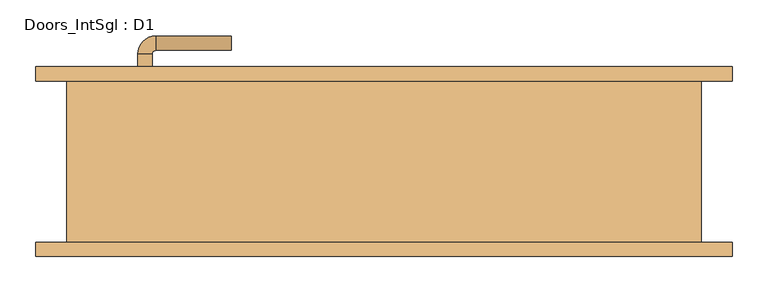
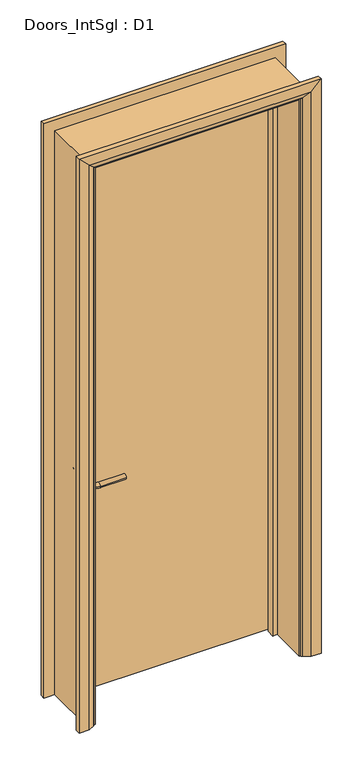
"""IFC4 building model written with IfcOpenShell, lengths in millimetres: door geometry, Doors_IntSgl : D1."""

from ifc_helpers import new_model, si_unit, point, frame, frame_2d, origin, place, context, project, spatial, polyline, circle_curve, ellipse_curve, trimmed, segment, composite_curve, outline, extrude, faceted_brep, source, transform, mapped, element, save
from ifc_brep_helpers import plane_surface, cylinder_surface, revolved_surface, advanced_brep


def doors_intsgl_d1_267d61ee(model_context):
    return source(origin(), model_context, "Body", "SolidModel", [
        advanced_brep(
        [(-343.0, 66.5, 900.0), (-323.0, 66.5, 900.0), (-323.0, 36.5, 900.0), (-343.0, 36.5, 900.0), (-318.0, 31.5, 900.0), (-318.0, 11.5, 900.0), (-213.0, 11.5, 900.0), (-213.0, 31.5, 900.0)],
        [
            (0, 1, circle_curve(frame((-333.0, 66.5, 900.0), z_axis=(0.0, 1.0, 0.0), x_axis=(1.0, 0.0, 0.0)), 10.0)),
            (1, 0, circle_curve(frame((-333.0, 66.5, 900.0), z_axis=(0.0, 1.0, 0.0), x_axis=(1.0, 0.0, 0.0)), 10.0)),
            (1, 2),
            (2, 3, circle_curve(frame((-333.0, 36.5, 900.0), z_axis=(0.0, 1.0, 0.0), x_axis=(1.0, 0.0, 0.0)), 10.0)),
            (3, 0),
            (3, 2, circle_curve(frame((-333.0, 36.5, 900.0), z_axis=(0.0, 1.0, 0.0), x_axis=(1.0, 0.0, 0.0)), 10.0)),
            (4, 5, circle_curve(frame((-318.0, 21.5, 900.0), z_axis=(-1.0, 0.0, 0.0), x_axis=(0.0, 1.0, 0.0)), 10.0)),
            (5, 3, circle_curve(frame((-318.0, 36.5, 900.0), z_axis=(0.0, 0.0, -1.0), x_axis=(-1.0, 0.0, 0.0)), 25.0)),
            (2, 4, circle_curve(frame((-318.0, 36.5, 900.0), z_axis=(0.0, 0.0, 1.0), x_axis=(-1.0, 0.0, 0.0)), 5.0)),
            (5, 4, circle_curve(frame((-318.0, 21.5, 900.0), z_axis=(-1.0, 0.0, 0.0), x_axis=(0.0, 1.0, 0.0)), 10.0)),
            (6, 7, circle_curve(frame((-213.0, 21.5, 900.0), z_axis=(1.0, 0.0, 0.0), x_axis=(0.0, 1.0, 0.0)), 10.0)),
            (7, 6, circle_curve(frame((-213.0, 21.5, 900.0), z_axis=(1.0, 0.0, 0.0), x_axis=(0.0, 1.0, 0.0)), 10.0)),
            (4, 7),
            (6, 5),
        ],
        [
            plane_surface(frame((-333.0, 66.5, 900.0), z_axis=(0.0, 1.0, 0.0), x_axis=(0.0, 0.0, 1.0))),
            cylinder_surface(frame((-333.0, 66.5, 900.0), z_axis=(0.0, 1.0, 0.0), x_axis=(1.0, 0.0, 0.0)), 10.0),
            revolved_surface(trimmed(ellipse_curve(frame((-333.0, 36.5, 900.0), z_axis=(0.0, -1.0, 0.0), x_axis=(1.0, 0.0, 0.0)), 10.0, 10.0), [point((-343.0, 36.5, 900.0))], [point((-323.0, 36.5, 900.0))], True, "CARTESIAN"), (-318.0, 36.5, 900.0), (0.0, 0.0, -1.0)),
            revolved_surface(trimmed(ellipse_curve(frame((-333.0, 36.5, 900.0), z_axis=(0.0, -1.0, 0.0), x_axis=(1.0, 0.0, 0.0)), 10.0, 10.0), [point((-323.0, 36.5, 900.0))], [point((-343.0, 36.5, 900.0))], True, "CARTESIAN"), (-318.0, 36.5, 900.0), (0.0, 0.0, -1.0)),
            plane_surface(frame((-213.0, 21.5, 900.0), z_axis=(1.0, 0.0, 0.0), x_axis=(0.0, 0.0, 1.0))),
            cylinder_surface(frame((-318.0, 21.5, 900.0), z_axis=(-1.0, 0.0, 0.0), x_axis=(0.0, 1.0, 0.0)), 10.0),
        ],
        [
            (0, [[1, 2]]),
            (1, [[3, 4, 5, -2]]),
            (1, [[-5, 6, -3, -1]]),
            (2, [[7, 8, -4, 9]]),
            (3, [[10, -9, -6, -8]]),
            (4, [[11, 12]]),
            (5, [[13, -11, 14, -7]]),
            (5, [[-14, -12, -13, -10]]),
        ],
    ),
        extrude(outline(composite_curve([segment(trimmed(circle_curve(frame_2d((900.0, -335.5)), 30.0), [point((900.0, -365.5))], [point((900.0, -305.5))], False, "CARTESIAN"), True, "CONTINUOUS"), segment(trimmed(circle_curve(frame_2d((900.0, -335.5)), 30.0), [point((900.0, -305.5))], [point((900.0, -365.5))], False, "CARTESIAN"), True, "CONTINUOUS")], self_intersect=False)), frame((0.0, 66.5, 0.0), z_axis=(0.0, 1.0, 0.0), x_axis=(0.0, 0.0, 1.0)), (0.0, 0.0, 1.0), 8.0),
        advanced_brep(
        [(-343.0, 120.5, 900.0), (-323.0, 120.5, 900.0), (-343.0, 150.5, 900.0), (-323.0, 150.5, 900.0), (-318.0, 155.5, 900.0), (-318.0, 175.5, 900.0), (-213.0, 175.5, 900.0), (-213.0, 155.5, 900.0)],
        [
            (0, 1, circle_curve(frame((-333.0, 120.5, 900.0), z_axis=(0.0, -1.0, 0.0), x_axis=(1.0, 0.0, 0.0)), 10.0)),
            (1, 0, circle_curve(frame((-333.0, 120.5, 900.0), z_axis=(0.0, -1.0, 0.0), x_axis=(1.0, 0.0, 0.0)), 10.0)),
            (0, 2),
            (2, 3, circle_curve(frame((-333.0, 150.5, 900.0), z_axis=(0.0, -1.0, 0.0), x_axis=(1.0, 0.0, 0.0)), 10.0)),
            (3, 1),
            (3, 2, circle_curve(frame((-333.0, 150.5, 900.0), z_axis=(0.0, -1.0, 0.0), x_axis=(1.0, 0.0, 0.0)), 10.0)),
            (4, 3, circle_curve(frame((-318.0, 150.5, 900.0), z_axis=(0.0, 0.0, 1.0), x_axis=(-1.0, 0.0, 0.0)), 5.0)),
            (2, 5, circle_curve(frame((-318.0, 150.5, 900.0), z_axis=(0.0, 0.0, -1.0), x_axis=(-1.0, 0.0, 0.0)), 25.0)),
            (5, 4, circle_curve(frame((-318.0, 165.5, 900.0), z_axis=(-1.0, 0.0, 0.0), x_axis=(0.0, -1.0, 0.0)), 10.0)),
            (4, 5, circle_curve(frame((-318.0, 165.5, 900.0), z_axis=(-1.0, 0.0, 0.0), x_axis=(0.0, -1.0, 0.0)), 10.0)),
            (6, 7, circle_curve(frame((-213.0, 165.5, 900.0), z_axis=(1.0, 0.0, 0.0), x_axis=(0.0, -1.0, 0.0)), 10.0)),
            (7, 6, circle_curve(frame((-213.0, 165.5, 900.0), z_axis=(1.0, 0.0, 0.0), x_axis=(0.0, -1.0, 0.0)), 10.0)),
            (5, 6),
            (7, 4),
        ],
        [
            plane_surface(frame((-333.0, 120.5, 900.0), z_axis=(0.0, -1.0, 0.0), x_axis=(0.0, 0.0, 1.0))),
            cylinder_surface(frame((-333.0, 120.5, 900.0), z_axis=(0.0, -1.0, 0.0), x_axis=(1.0, 0.0, 0.0)), 10.0),
            revolved_surface(trimmed(ellipse_curve(frame((-333.0, 150.5, 900.0), z_axis=(0.0, -1.0, 0.0), x_axis=(1.0, 0.0, 0.0)), 10.0, 10.0), [point((-343.0, 150.5, 900.0))], [point((-323.0, 150.5, 900.0))], True, "CARTESIAN"), (-318.0, 150.5, 900.0), (0.0, 0.0, -1.0)),
            revolved_surface(trimmed(ellipse_curve(frame((-333.0, 150.5, 900.0), z_axis=(0.0, -1.0, 0.0), x_axis=(1.0, 0.0, 0.0)), 10.0, 10.0), [point((-323.0, 150.5, 900.0))], [point((-343.0, 150.5, 900.0))], True, "CARTESIAN"), (-318.0, 150.5, 900.0), (0.0, 0.0, -1.0)),
            plane_surface(frame((-213.0, 165.5, 900.0), z_axis=(1.0, 0.0, 0.0), x_axis=(0.0, 0.0, 1.0))),
            cylinder_surface(frame((-318.0, 165.5, 900.0), z_axis=(-1.0, 0.0, 0.0), x_axis=(0.0, -1.0, 0.0)), 10.0),
        ],
        [
            (0, [[1, 2]]),
            (1, [[-1, 3, 4, 5]]),
            (1, [[-2, -5, 6, -3]]),
            (2, [[7, -4, 8, 9]]),
            (3, [[-8, -6, -7, 10]]),
            (4, [[11, 12]]),
            (5, [[-9, 13, -12, 14]]),
            (5, [[-10, -14, -11, -13]]),
        ],
    ),
        extrude(outline(composite_curve([segment(trimmed(circle_curve(frame_2d((900.0, -335.5)), 30.0), [point((900.0, -365.5))], [point((900.0, -305.5))], False, "CARTESIAN"), True, "CONTINUOUS"), segment(trimmed(circle_curve(frame_2d((900.0, -335.5)), 30.0), [point((900.0, -305.5))], [point((900.0, -365.5))], False, "CARTESIAN"), True, "CONTINUOUS")], self_intersect=False)), frame((0.0, 112.5, 0.0), z_axis=(0.0, 1.0, 0.0), x_axis=(0.0, 0.0, 1.0)), (0.0, 0.0, 1.0), 8.0),
        extrude(outline(polyline([(408.0, 74.5), (-408.0, 74.5), (-408.0, 112.5), (408.0, 112.5), (408.0, 74.5)])), frame((0.0, 0.0, 8.0), z_axis=(0.0, 0.0, 1.0), x_axis=(1.0, 0.0, 0.0)), (0.0, 0.0, 1.0), 2350.0),
        faceted_brep([(-410.0, 112.5, 0.0), (-410.0, -112.5, 0.0), (-442.0, -112.5, 0.0), (-442.0, 112.5, 0.0), (-410.0, 112.5, 2360.0), (-410.0, -112.5, 2360.0), (-442.0, -112.5, 2392.0), (-442.0, 112.5, 2392.0), (410.0, 112.5, 0.0), (442.0, 112.5, 0.0), (442.0, -112.5, 0.0), (410.0, -112.5, 0.0), (410.0, 112.5, 2360.0), (442.0, 112.5, 2392.0), (442.0, -112.5, 2392.0), (410.0, -112.5, 2360.0)], [[[0, 1, 2, 3]], [[1, 0, 4, 5]], [[2, 1, 5, 6]], [[3, 2, 6, 7]], [[0, 3, 7, 4]], [[8, 9, 10, 11]], [[12, 13, 9, 8]], [[13, 14, 10, 9]], [[14, 15, 11, 10]], [[15, 12, 8, 11]], [[5, 4, 12, 15]], [[6, 5, 15, 14]], [[7, 6, 14, 13]], [[4, 7, 13, 12]]]),
        advanced_brep(
        [(-485.0, -132.5, 0.0), (-485.0, -112.5, 0.0), (-415.0, -112.5, 0.0), (-419.0, -118.5, 0.0), (-445.0, -132.5, 0.0), (-485.0, -132.5, 2435.0), (-485.0, -112.5, 2435.0), (-415.0, -112.5, 2365.0), (-419.0, -118.5, 2369.0), (-445.0, -132.5, 2395.0), (485.0, -132.5, 0.0), (445.0, -132.5, 0.0), (419.0, -118.5, 0.0), (415.0, -112.5, 0.0), (485.0, -112.5, 0.0), (485.0, -132.5, 2435.0), (445.0, -132.5, 2395.0), (419.0, -118.5, 2369.0), (415.0, -112.5, 2365.0), (485.0, -112.5, 2435.0)],
        [
            (0, 1),
            (1, 2),
            (2, 3, circle_curve(frame((-423.0, -111.5, 0.0), z_axis=(0.0, 0.0, -1.0), x_axis=(-1.0, 0.0, 0.0)), 8.0622577)),
            (3, 4),
            (4, 0),
            (0, 5),
            (5, 6),
            (6, 1),
            (6, 7),
            (7, 2),
            (7, 8, ellipse_curve(frame((-423.0, -111.5, 2373.0), z_axis=(-0.7071067811865475, 0.0, -0.7071067811865475), x_axis=(0.7071067811865474, 0.0, -0.7071067811865476)), 11.4017543, 8.0622577)),
            (8, 3),
            (8, 9),
            (9, 4),
            (9, 5),
            (10, 11),
            (11, 12),
            (12, 13, circle_curve(frame((423.0, -111.5, 0.0), z_axis=(0.0, 0.0, -1.0), x_axis=(1.0, 0.0, 0.0)), 8.0622577)),
            (13, 14),
            (14, 10),
            (15, 16),
            (16, 11),
            (10, 15),
            (16, 17),
            (17, 12),
            (17, 18, ellipse_curve(frame((423.0, -111.5, 2373.0), z_axis=(0.7071067811865475, 0.0, -0.7071067811865475), x_axis=(0.7071067811865474, 0.0, 0.7071067811865476)), 11.4017543, 8.0622577)),
            (18, 13),
            (18, 19),
            (19, 14),
            (19, 15),
            (5, 15),
            (19, 6),
            (18, 7),
            (17, 8),
            (16, 9),
        ],
        [
            plane_surface(frame((-415.0, -185.3010989, 0.0), z_axis=(0.0, 0.0, -1.0), x_axis=(1.0, 0.0, 0.0))),
            plane_surface(frame((-485.0, -132.5, 0.0), z_axis=(-1.0, 0.0, 0.0), x_axis=(0.0, 0.0, 1.0))),
            plane_surface(frame((-485.0, -112.5, 0.0), z_axis=(0.0, 1.0, 0.0), x_axis=(0.0, 0.0, 1.0))),
            cylinder_surface(frame((-423.0, -111.5, 0.0), z_axis=(0.0, 0.0, -1.0), x_axis=(-1.0, 0.0, 0.0)), 8.0622577),
            plane_surface(frame((-419.0, -118.5, 0.0), z_axis=(0.4740998230350183, -0.8804710999221749, 0.0), x_axis=(0.0, 0.0, 1.0))),
            plane_surface(frame((-445.0, -132.5, 0.0), z_axis=(0.0, -1.0, 0.0), x_axis=(0.0, 0.0, 1.0))),
            plane_surface(frame((415.0, -185.3010989, 0.0), z_axis=(0.0, 0.0, -1.0), x_axis=(-1.0, 0.0, 0.0))),
            plane_surface(frame((445.0, -132.5, 2395.0), z_axis=(0.0, -1.0, 0.0), x_axis=(0.0, 0.0, -1.0))),
            plane_surface(frame((419.0, -118.5, 2369.0), z_axis=(-0.4740998230350183, -0.8804710999221749, 0.0), x_axis=(0.0, 0.0, -1.0))),
            cylinder_surface(frame((423.0, -111.5, 2365.0), z_axis=(0.0, 0.0, 1.0), x_axis=(1.0, 0.0, 0.0)), 8.0622577),
            plane_surface(frame((485.0, -112.5, 2435.0), z_axis=(0.0, 1.0, 0.0), x_axis=(0.0, 0.0, -1.0))),
            plane_surface(frame((485.0, -132.5, 2435.0), z_axis=(1.0, 0.0, 0.0), x_axis=(0.0, 0.0, -1.0))),
            plane_surface(frame((-485.0, -132.5, 2435.0), z_axis=(0.0, 0.0, 1.0), x_axis=(1.0, 0.0, 0.0))),
            plane_surface(frame((-485.0, -112.5, 2435.0), z_axis=(0.0, 1.0, 0.0), x_axis=(1.0, 0.0, 0.0))),
            cylinder_surface(frame((-415.0, -111.5, 2373.0), z_axis=(-1.0, 0.0, 0.0), x_axis=(0.0, 0.0, 1.0)), 8.0622577),
            plane_surface(frame((-419.0, -118.5, 2369.0), z_axis=(0.0, -0.8804710999221749, -0.4740998230350183), x_axis=(1.0, 0.0, 0.0))),
            plane_surface(frame((-445.0, -132.5, 2395.0), z_axis=(0.0, -1.0, 0.0), x_axis=(1.0, 0.0, 0.0))),
        ],
        [
            (0, [[1, 2, 3, 4, 5]]),
            (1, [[-1, 6, 7, 8]]),
            (2, [[-2, -8, 9, 10]]),
            (3, [[-3, -10, 11, 12]]),
            (4, [[-4, -12, 13, 14]]),
            (5, [[-5, -14, 15, -6]]),
            (6, [[16, 17, 18, 19, 20]]),
            (7, [[21, 22, -16, 23]]),
            (8, [[24, 25, -17, -22]]),
            (9, [[26, 27, -18, -25]]),
            (10, [[28, 29, -19, -27]]),
            (11, [[30, -23, -20, -29]]),
            (12, [[-7, 31, -30, 32]]),
            (13, [[-9, -32, -28, 33]]),
            (14, [[-11, -33, -26, 34]]),
            (15, [[-13, -34, -24, 35]]),
            (16, [[-15, -35, -21, -31]]),
        ],
    ),
        extrude(outline(polyline([(0.0, -410.0), (0.0, -391.0), (2341.0, -391.0), (2341.0, 391.0), (0.0, 391.0), (0.0, 410.0), (2360.0, 410.0), (2360.0, -410.0), (0.0, -410.0)])), frame((0.0, 40.5, 0.0), z_axis=(0.0, 1.0, 0.0), x_axis=(0.0, 0.0, 1.0)), (0.0, 0.0, 1.0), 32.0),
        advanced_brep(
        [(485.0, 132.5, 0.0), (485.0, 112.5, 0.0), (415.0, 112.5, 0.0), (419.0, 118.5, 0.0), (445.0, 132.5, 0.0), (485.0, 132.5, 2435.0), (485.0, 112.5, 2435.0), (-485.0, 112.5, 2435.0), (-485.0, 112.5, 0.0), (-415.0, 112.5, 0.0), (-415.0, 112.5, 2365.0), (415.0, 112.5, 2365.0), (419.0, 118.5, 2369.0), (445.0, 132.5, 2395.0), (-445.0, 132.5, 2395.0), (-445.0, 132.5, 0.0), (-485.0, 132.5, 0.0), (-485.0, 132.5, 2435.0), (-419.0, 118.5, 0.0), (-419.0, 118.5, 2369.0)],
        [
            (0, 1),
            (1, 2),
            (2, 3, circle_curve(frame((423.0, 111.5, 0.0), z_axis=(0.0, 0.0, -1.0), x_axis=(1.0, 0.0, 0.0)), 8.0622577)),
            (3, 4),
            (4, 0),
            (0, 5),
            (5, 6),
            (6, 1),
            (6, 7),
            (7, 8),
            (8, 9),
            (9, 10),
            (10, 11),
            (11, 2),
            (11, 12, ellipse_curve(frame((423.0, 111.5, 2373.0), z_axis=(0.7071067811865475, 0.0, -0.7071067811865475), x_axis=(-0.7071067811865474, 0.0, -0.7071067811865476)), 11.4017543, 8.0622577)),
            (12, 3),
            (12, 13),
            (13, 4),
            (13, 14),
            (14, 15),
            (15, 16),
            (16, 17),
            (17, 5),
            (7, 17),
            (16, 8),
            (15, 18),
            (18, 9, circle_curve(frame((-423.0, 111.5, 0.0), z_axis=(0.0, 0.0, -1.0), x_axis=(-1.0, 0.0, 0.0)), 8.0622577)),
            (19, 10, ellipse_curve(frame((-423.0, 111.5, 2373.0), z_axis=(-0.7071067811865475, 0.0, -0.7071067811865475), x_axis=(-0.7071067811865474, 0.0, 0.7071067811865476)), 11.4017543, 8.0622577)),
            (18, 19),
            (14, 19),
            (19, 12),
        ],
        [
            plane_surface(frame((415.0, 112.5, 0.0), z_axis=(0.0, 0.0, -1.0), x_axis=(0.0, -1.0, 0.0))),
            plane_surface(frame((485.0, 132.5, 0.0), z_axis=(1.0, 0.0, 0.0), x_axis=(0.0, 0.0, 1.0))),
            plane_surface(frame((485.0, 112.5, 0.0), z_axis=(0.0, -1.0, 0.0), x_axis=(0.0, 0.0, 1.0))),
            cylinder_surface(frame((423.0, 111.5, 0.0), z_axis=(0.0, 0.0, -1.0), x_axis=(1.0, 0.0, 0.0)), 8.0622577),
            plane_surface(frame((419.0, 118.5, 0.0), z_axis=(-0.4740998230350126, 0.880471099922178, 0.0), x_axis=(0.0, 0.0, 1.0))),
            plane_surface(frame((445.0, 132.5, 0.0), z_axis=(0.0, 1.0, 0.0), x_axis=(0.0, 0.0, 1.0))),
            plane_surface(frame((-485.0, 132.5, 2435.0), z_axis=(-1.0, 0.0, 0.0), x_axis=(0.0, 0.0, -1.0))),
            plane_surface(frame((-415.0, 112.5, 0.0), z_axis=(0.0, 0.0, -1.0), x_axis=(0.0, -1.0, 0.0))),
            cylinder_surface(frame((-423.0, 111.5, 2365.0), z_axis=(0.0, 0.0, 1.0), x_axis=(-1.0, 0.0, 0.0)), 8.0622577),
            plane_surface(frame((-419.0, 118.5, 2369.0), z_axis=(0.47409982303501824, 0.8804710999221749, 0.0), x_axis=(0.0, 0.0, -1.0))),
            plane_surface(frame((485.0, 132.5, 2435.0), z_axis=(0.0, 0.0, 1.0), x_axis=(-1.0, 0.0, 0.0))),
            cylinder_surface(frame((415.0, 111.5, 2373.0), z_axis=(1.0, 0.0, 0.0), x_axis=(0.0, 0.0, 1.0)), 8.0622577),
            plane_surface(frame((419.0, 118.5, 2369.0), z_axis=(0.0, 0.8804710999221764, -0.4740998230350154), x_axis=(-1.0, 0.0, 0.0))),
        ],
        [
            (0, [[1, 2, 3, 4, 5]]),
            (1, [[-1, 6, 7, 8]]),
            (2, [[-2, -8, 9, 10, 11, 12, 13, 14]]),
            (3, [[-3, -14, 15, 16]]),
            (4, [[-4, -16, 17, 18]]),
            (5, [[-5, -18, 19, 20, 21, 22, 23, -6]]),
            (6, [[24, -22, 25, -10]]),
            (7, [[-21, 26, 27, -11, -25]]),
            (8, [[28, -12, -27, 29]]),
            (9, [[30, -29, -26, -20]]),
            (10, [[-7, -23, -24, -9]]),
            (11, [[-15, -13, -28, 31]]),
            (12, [[-17, -31, -30, -19]]),
        ],
    ),
    ])


if __name__ == "__main__":
    model = new_model("IFC4")
    model_context = context("Model", 3, world=origin())
    ifc_project = project(units=[si_unit("LENGTHUNIT", "METRE", prefix="MILLI")], contexts=[model_context])
    site = spatial("IfcSite", under=ifc_project)
    building = spatial("IfcBuilding", under=site)
    placement = place(None, origin())
    doors_intsgl_d1_shape = doors_intsgl_d1_267d61ee(model_context)
    element("IfcDoor", 1, ObjectType="Doors_IntSgl : D1", at=placement, inside=building, context=model_context, shape_type="MappedRepresentation", body=[
        mapped(doors_intsgl_d1_shape, transform((0.0, 0.0, 0.0), x_axis=(1.0, 0.0, 0.0), y_axis=(0.0, 1.0, 0.0), z_axis=(0.0, 0.0, 1.0))),
    ])
    save(model, "model.ifc")

# Revit data of these elements
# Type "Doors_IntSgl : D1"
#   Type Mark = "51"
#   Type Comments = "Internal Single"
#   Operation = "SingleSwingRight"
#   Manufacturer = "Revit"
#   Keynote = "L20"
#   Description = "Internal Single Door"
#   Analytic Construction = "Metal"
#   UnderCut = 8 mm
#   Tolerance = 2 mm
#   Thickness = 38 mm
#   Thermal Resistance (R) = 0.270117 (m²·K)/W
#   Structural Tolerance = 8 mm
#   StopDepth = 32 mm
#   Stop Thickness = 19 mm
#   Rough Width = 900 mm
#   Rough Height = 2400 mm
#   Height to Top Lock Rail = 1000 mm
#   Heat Transfer Coefficient (U) = 3.7021 W/(m²·K)
#   Handle Z Distance = 900 mm
#   Handle X Distance = 75 mm
#   Frame Thickness = 32 mm
#   Door Panel Width = 816 mm
#   Door Panel Thickness = 38 mm
#   Door Panel Offset = 0 mm
#   Height = 2400 mm
#   Width = 900 mm
#   Door Panel Height = 2350 mm
#   Architrave Setback = 5 mm
#   Vis - Ironmongery = yes
#   Define Thermal Properties by = 1
#   Material Ironmongery = Door - Handle
#   Material Frame = Door - Frame/Mullion (1)
#   Material Door = Door - Panel
#   Material Architrave = Door - Architrave
#   Visual Light Transmittance = 0
#   Solar Heat Gain Coefficient = 0
#   Function = (empty or 0)
#   Wall Closure = (empty or 0)
# Element 1 (IfcDoor, "Doors_IntSgl : D1")
#   Materials on its faces: "Door - Architrave", "Door - Handle", "Door - Frame/Mullion (1)", "Door - Panel"
# Materials
#   "Door - Handle": colour RGB 0 0 0, transparency 0, Keynote = "P21", Cost = 0
#   "Door - Frame/Mullion (1)": class "Wood", colour RGB 212 179 113, transparency 0, Keynote = "L20", Cost = 0
#   "Door - Panel": class "Wood", colour RGB 210 159 95, transparency 0, Keynote = "L20", Cost = 0
#   "Door - Architrave": class "Wood", colour RGB 154 90 5, transparency 0, Keynote = "P20", Cost = 0
